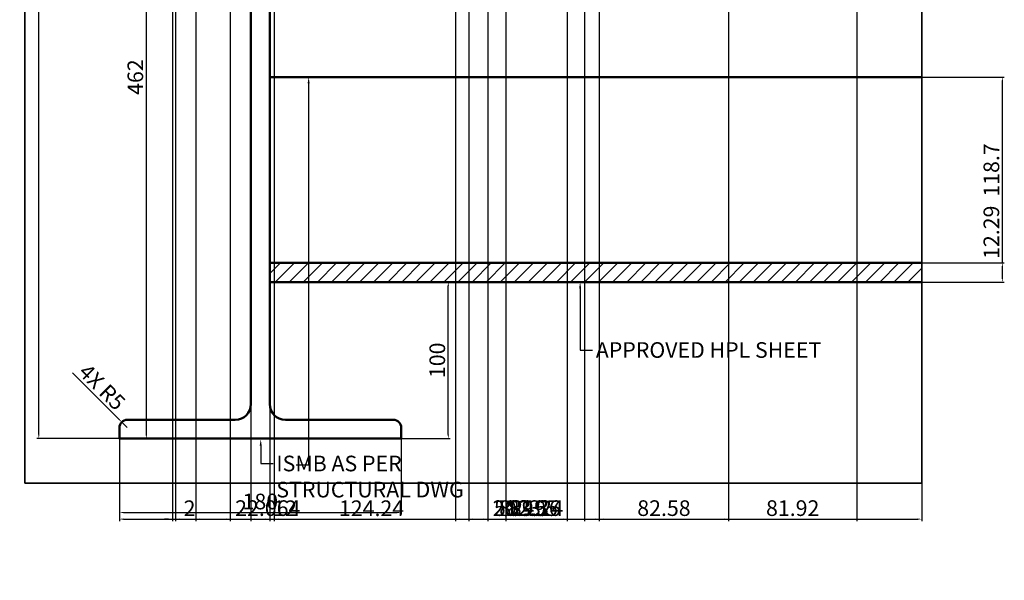
# Model space of a CAD drawing. Units: millimetres. Extents: x 1791 to 2420, y 1225 to 2361.
# Tile 1 of 4: x 1791 to 2420, y 1225 to 1583. Entities that reach past the tile are written whole.
import ezdxf
from ezdxf import colors
from ezdxf.entities.mleader import LeaderData, LeaderLine
from ezdxf.math import Vec2, Vec3

# ---------------------------------------------------------------- set-up
doc = ezdxf.new("R2010")
doc.units = ezdxf.units.MM
for name, color, linetype, lineweight in [('A-ANNO-DIMS', 2, 'Continuous', 18), ('A-ANNO-TEXT', 7, 'Continuous', 18), ('A-ANNO-TTLB', 7, 'Continuous', 35), ('A-DETL-PATT', 8, 'Continuous', 13), ('S-BEAM', 1, 'Continuous', 50)]:
    doc.layers.add(name, color=color, linetype=linetype, lineweight=lineweight)
doc.styles.get("Standard").update_dxf_attribs({"font": 'arial.ttf'})
doc.dimstyles.new('ISO-25', dxfattribs={"dimtxt": 10, "dimasz": 2.5, "dimexe": 1.25, "dimexo": 0.625, "dimtad": 1, "dimdec": 1, "dimtxsty": 'Standard', "dimcen": 2.5, "dimadec": 0, "dimazin": 0, "dimtfac": 1, "dimtdec": 1, "dimtmove": 0, "dimatfit": 3, "dimfxl": 1, "dimarcsym": 0})

# ---------------------------------------------------------------- blocks, each defined once
blk = doc.blocks.new('*D3')
at = {"layer": 'A-ANNO-DIMS', "color": 0, "lineweight": -2, "transparency": 16777216}
for p, q in [((1860.7, 1777.42), (1873.17, 1777.42)), ((1871.92, 1317.92), (1871.92, 1774.92)), ((1860.7, 1315.42), (1873.17, 1315.42))]:
    blk.add_line(p, q, dxfattribs=at)
at = {"layer": 'A-ANNO-DIMS', "color": 0, "transparency": 16777216}
for points in [[(1871.5, 1774.92), (1872.34, 1774.92), (1871.92, 1777.42)], [(1871.5, 1317.92), (1872.34, 1317.92), (1871.92, 1315.42)]]:
    blk.add_solid(points, dxfattribs=at)
at = {"layer": 'Defpoints', "color": 0, "transparency": 16777216}
for p in [(1860.08, 1777.42), (1871.92, 1777.42), (1860.08, 1315.42)]:
    blk.add_point(p, dxfattribs=at)
at = {"layer": 'A-ANNO-DIMS', "color": 0, "transparency": 16777216, "insert": (1866.19, 1546.42), "char_height": 10, "attachment_point": 5, "rotation": 90}
blk.add_mtext('462', dxfattribs=at)
blk = doc.blocks.new('*D5')
at = {"layer": 'A-ANNO-DIMS', "color": 0, "lineweight": -2, "transparency": 16777216}
for p, q in [((1854.73, 1314.8), (1854.73, 1266.91)), ((2034.73, 1314.8), (2034.73, 1266.91)), ((1857.23, 1268.16), (2032.23, 1268.16))]:
    blk.add_line(p, q, dxfattribs=at)
at = {"layer": 'A-ANNO-DIMS', "color": 0, "transparency": 16777216}
for points in [[(1857.23, 1268.58), (1857.23, 1267.74), (1854.73, 1268.16)], [(2032.23, 1268.58), (2032.23, 1267.74), (2034.73, 1268.16)]]:
    blk.add_solid(points, dxfattribs=at)
at = {"layer": 'Defpoints', "color": 0, "transparency": 16777216}
for p in [(1854.73, 1315.42), (2034.73, 1315.42), (2034.73, 1268.16)]:
    blk.add_point(p, dxfattribs=at)
at = {"layer": 'A-ANNO-DIMS', "color": 0, "transparency": 16777216, "insert": (1944.73, 1273.89), "char_height": 10, "attachment_point": 5}
blk.add_mtext('180', dxfattribs=at)
blk = doc.blocks.new('*D6')
at = {"layer": 'A-ANNO-DIMS', "color": 0, "lineweight": -2, "transparency": 16777216}
for p, q in [((2035.35, 1415.42), (2066.04, 1415.42)), ((2064.79, 1317.92), (2064.79, 1412.92)), ((2035.35, 1315.42), (2066.04, 1315.42))]:
    blk.add_line(p, q, dxfattribs=at)
at = {"layer": 'A-ANNO-DIMS', "color": 0, "transparency": 16777216}
for points in [[(2064.38, 1412.92), (2065.21, 1412.92), (2064.79, 1415.42)], [(2064.38, 1317.92), (2065.21, 1317.92), (2064.79, 1315.42)]]:
    blk.add_solid(points, dxfattribs=at)
at = {"layer": 'Defpoints', "color": 0, "transparency": 16777216}
for p in [(2034.73, 1415.42), (2064.79, 1415.42), (2034.73, 1315.42)]:
    blk.add_point(p, dxfattribs=at)
at = {"layer": 'A-ANNO-DIMS', "color": 0, "transparency": 16777216, "insert": (2059.06, 1365.42), "char_height": 10, "attachment_point": 5, "rotation": 90}
blk.add_mtext('100', dxfattribs=at)
blk = doc.blocks.new('*D10')
at = {"layer": 'A-ANNO-DIMS', "color": 0, "lineweight": -2, "transparency": 16777216}
for p, q in [((2367.22, 1414.8), (2367.22, 1262.67)), ((1854.73, 1314.8), (1854.73, 1262.67)), ((1857.23, 1263.92), (2364.72, 1263.92))]:
    blk.add_line(p, q, dxfattribs=at)
at = {"layer": 'A-ANNO-DIMS', "color": 0, "transparency": 16777216}
for points in [[(1857.23, 1264.34), (1857.23, 1263.5), (1854.73, 1263.92)], [(2364.72, 1264.34), (2364.72, 1263.5), (2367.22, 1263.92)]]:
    blk.add_solid(points, dxfattribs=at)
at = {"layer": 'Defpoints', "color": 0, "transparency": 16777216}
for p in [(2367.22, 1415.42), (1854.73, 1315.42), (2367.22, 1263.92)]:
    blk.add_point(p, dxfattribs=at)
at = {"layer": 'A-ANNO-DIMS', "color": 0, "transparency": 16777216, "insert": (2110.97, 1269.65), "char_height": 10, "attachment_point": 5}
blk.add_mtext('512.5', dxfattribs=at)
blk = doc.blocks.new('*D11')
at = {"layer": 'A-ANNO-DIMS', "color": 0, "lineweight": -2, "transparency": 16777216}
for p, q in [((1894.37, 2284.98), (1801.98, 2284.98)), ((1803.23, 1317.92), (1803.23, 2282.48)), ((1854.1, 1315.42), (1801.98, 1315.42))]:
    blk.add_line(p, q, dxfattribs=at)
at = {"layer": 'A-ANNO-DIMS', "color": 0, "transparency": 16777216}
for points in [[(1802.81, 2282.48), (1803.64, 2282.48), (1803.23, 2284.98)], [(1802.81, 1317.92), (1803.64, 1317.92), (1803.23, 1315.42)]]:
    blk.add_solid(points, dxfattribs=at)
at = {"layer": 'Defpoints', "color": 0, "transparency": 16777216}
for p in [(1803.23, 2284.98), (1895, 2284.98), (1854.73, 1315.42)]:
    blk.add_point(p, dxfattribs=at)
at = {"layer": 'A-ANNO-DIMS', "color": 0, "transparency": 16777216, "insert": (1797.5, 1800.2), "char_height": 10, "attachment_point": 5, "rotation": 90}
blk.add_mtext('969.6', dxfattribs=at)
blk = doc.blocks.new('*D16')
at = {"layer": 'A-ANNO-DIMS', "color": 0, "lineweight": -2, "transparency": 16777216}
for p, q in [((1888.61, 1776.8), (1888.61, 1262.67)), ((1890.61, 1778.8), (1890.61, 1262.67)), ((1886.11, 1263.92), (1883.61, 1263.92)), ((1888.61, 1263.92), (1890.61, 1263.92)), ((1893.11, 1263.92), (1903.49, 1263.92))]:
    blk.add_line(p, q, dxfattribs=at)
at = {"layer": 'A-ANNO-DIMS', "color": 0, "transparency": 16777216}
for points in [[(1886.11, 1264.34), (1886.11, 1263.5), (1888.61, 1263.92)], [(1893.11, 1264.34), (1893.11, 1263.5), (1890.61, 1263.92)]]:
    blk.add_solid(points, dxfattribs=at)
at = {"layer": 'Defpoints', "color": 0, "transparency": 16777216}
for p in [(1888.61, 1777.42), (1890.61, 1779.42), (1890.61, 1263.92)]:
    blk.add_point(p, dxfattribs=at)
at = {"layer": 'A-ANNO-DIMS', "color": 0, "transparency": 16777216, "insert": (1899.55, 1269.57), "char_height": 10, "attachment_point": 5}
blk.add_mtext('2', dxfattribs=at)
blk = doc.blocks.new('*D17')
at = {"layer": 'A-ANNO-DIMS', "color": 0, "lineweight": -2, "transparency": 16777216}
for p, q in [((1903.46, 1791.65), (1903.46, 1262.67)), ((1925.53, 1791.65), (1925.53, 1262.67)), ((1905.96, 1263.92), (1923.03, 1263.92)), ((1925.53, 1263.92), (1970.92, 1263.92))]:
    blk.add_line(p, q, dxfattribs=at)
at = {"layer": 'A-ANNO-DIMS', "color": 0, "transparency": 16777216}
for points in [[(1905.96, 1264.34), (1905.96, 1263.5), (1903.46, 1263.92)], [(1923.03, 1264.34), (1923.03, 1263.5), (1925.53, 1263.92)]]:
    blk.add_solid(points, dxfattribs=at)
at = {"layer": 'Defpoints', "color": 0, "transparency": 16777216}
for p in [(1903.46, 1792.27), (1925.53, 1792.27), (1925.53, 1263.92)]:
    blk.add_point(p, dxfattribs=at)
at = {"layer": 'A-ANNO-DIMS', "color": 0, "transparency": 16777216, "insert": (1949.47, 1269.65), "char_height": 10, "attachment_point": 5}
blk.add_mtext('22.064', dxfattribs=at)
blk = doc.blocks.new('*D20')
at = {"layer": 'A-ANNO-DIMS', "color": 0, "lineweight": -2, "transparency": 16777216}
for p, q in [((1938.73, 1336.8), (1938.73, 1262.67)), ((1950.73, 1336.8), (1950.73, 1262.67)), ((1941.23, 1263.92), (1948.23, 1263.92)), ((1950.73, 1263.92), (1967.76, 1263.92))]:
    blk.add_line(p, q, dxfattribs=at)
at = {"layer": 'A-ANNO-DIMS', "color": 0, "transparency": 16777216}
for points in [[(1941.23, 1264.34), (1941.23, 1263.5), (1938.73, 1263.92)], [(1948.23, 1264.34), (1948.23, 1263.5), (1950.73, 1263.92)]]:
    blk.add_solid(points, dxfattribs=at)
at = {"layer": 'Defpoints', "color": 0, "transparency": 16777216}
for p in [(1938.73, 1337.42), (1950.73, 1337.42), (1950.73, 1263.92)]:
    blk.add_point(p, dxfattribs=at)
at = {"layer": 'A-ANNO-DIMS', "color": 0, "transparency": 16777216, "insert": (1960.49, 1269.57), "char_height": 10, "attachment_point": 5}
blk.add_mtext('12', dxfattribs=at)
blk = doc.blocks.new('*D29')
at = {"layer": 'A-ANNO-DIMS', "color": 0, "lineweight": -2, "transparency": 16777216}
for p, q in [((2069.49, 1724.43), (2069.49, 1262.67)), ((2089.99, 1724.43), (2089.99, 1262.67)), ((2071.99, 1263.92), (2087.49, 1263.92)), ((2089.99, 1263.92), (2135.5, 1263.92))]:
    blk.add_line(p, q, dxfattribs=at)
at = {"layer": 'A-ANNO-DIMS', "color": 0, "transparency": 16777216}
for points in [[(2071.99, 1264.34), (2071.99, 1263.5), (2069.49, 1263.92)], [(2087.49, 1264.34), (2087.49, 1263.5), (2089.99, 1263.92)]]:
    blk.add_solid(points, dxfattribs=at)
at = {"layer": 'Defpoints', "color": 0, "transparency": 16777216}
for p in [(2069.49, 1725.06), (2089.99, 1725.06), (2089.99, 1263.92)]:
    blk.add_point(p, dxfattribs=at)
at = {"layer": 'A-ANNO-DIMS', "color": 0, "transparency": 16777216, "insert": (2113.99, 1269.65), "char_height": 10, "attachment_point": 5}
blk.add_mtext('20.495', dxfattribs=at)
blk = doc.blocks.new('*D30')
at = {"layer": 'A-ANNO-DIMS', "color": 0, "lineweight": -2, "transparency": 16777216}
for p, q in [((2069.49, 1724.43), (2069.49, 1262.67)), ((2151.78, 1724.43), (2151.78, 1262.67)), ((2071.99, 1263.92), (2149.28, 1263.92))]:
    blk.add_line(p, q, dxfattribs=at)
at = {"layer": 'A-ANNO-DIMS', "color": 0, "transparency": 16777216}
for points in [[(2071.99, 1264.34), (2071.99, 1263.5), (2069.49, 1263.92)], [(2149.28, 1264.34), (2149.28, 1263.5), (2151.78, 1263.92)]]:
    blk.add_solid(points, dxfattribs=at)
at = {"layer": 'Defpoints', "color": 0, "transparency": 16777216}
for p in [(2069.49, 1725.06), (2151.78, 1725.06), (2151.78, 1263.92)]:
    blk.add_point(p, dxfattribs=at)
at = {"layer": 'A-ANNO-DIMS', "color": 0, "transparency": 16777216, "insert": (2110.64, 1269.65), "char_height": 10, "attachment_point": 5}
blk.add_mtext('82.3', dxfattribs=at)
blk = doc.blocks.new('*D31')
at = {"layer": 'A-ANNO-DIMS', "color": 0, "lineweight": -2, "transparency": 16777216}
for p, q in [((2101.6, 1745.71), (2101.6, 1262.67)), ((2140.84, 1745.71), (2140.84, 1262.67)), ((2104.1, 1263.92), (2138.34, 1263.92))]:
    blk.add_line(p, q, dxfattribs=at)
at = {"layer": 'A-ANNO-DIMS', "color": 0, "transparency": 16777216}
for points in [[(2104.1, 1264.34), (2104.1, 1263.5), (2101.6, 1263.92)], [(2138.34, 1264.34), (2138.34, 1263.5), (2140.84, 1263.92)]]:
    blk.add_solid(points, dxfattribs=at)
at = {"layer": 'Defpoints', "color": 0, "transparency": 16777216}
for p in [(2101.6, 1746.33), (2140.84, 1746.33), (2140.84, 1263.92)]:
    blk.add_point(p, dxfattribs=at)
at = {"layer": 'A-ANNO-DIMS', "color": 0, "transparency": 16777216, "insert": (2121.22, 1269.65), "char_height": 10, "attachment_point": 5}
blk.add_mtext('39.24', dxfattribs=at)
blk = doc.blocks.new('*D32')
at = {"layer": 'A-ANNO-DIMS', "color": 0, "lineweight": -2, "transparency": 16777216}
for p, q in [((1953.66, 1761.87), (1953.66, 1262.67)), ((2077.9, 1766.79), (2077.9, 1262.67)), ((1956.16, 1263.92), (2075.4, 1263.92))]:
    blk.add_line(p, q, dxfattribs=at)
at = {"layer": 'A-ANNO-DIMS', "color": 0, "transparency": 16777216}
for points in [[(1956.16, 1264.34), (1956.16, 1263.5), (1953.66, 1263.92)], [(2075.4, 1264.34), (2075.4, 1263.5), (2077.9, 1263.92)]]:
    blk.add_solid(points, dxfattribs=at)
at = {"layer": 'Defpoints', "color": 0, "transparency": 16777216}
for p in [(2077.9, 1767.42), (1953.66, 1762.49), (2077.9, 1263.92)]:
    blk.add_point(p, dxfattribs=at)
at = {"layer": 'A-ANNO-DIMS', "color": 0, "transparency": 16777216, "insert": (2015.78, 1269.57), "char_height": 10, "attachment_point": 5}
blk.add_mtext('124.24', dxfattribs=at)
blk = doc.blocks.new('*D33')
at = {"layer": 'A-ANNO-DIMS', "color": 0, "lineweight": -2, "transparency": 16777216}
for p, q in [((2077.9, 1766.79), (2077.9, 1262.67)), ((2161.26, 1766.79), (2161.26, 1262.67)), ((2080.4, 1263.92), (2158.76, 1263.92))]:
    blk.add_line(p, q, dxfattribs=at)
at = {"layer": 'A-ANNO-DIMS', "color": 0, "transparency": 16777216}
for points in [[(2080.4, 1264.34), (2080.4, 1263.5), (2077.9, 1263.92)], [(2158.76, 1264.34), (2158.76, 1263.5), (2161.26, 1263.92)]]:
    blk.add_solid(points, dxfattribs=at)
at = {"layer": 'Defpoints', "color": 0, "transparency": 16777216}
for p in [(2077.9, 1767.42), (2161.26, 1767.42), (2161.26, 1263.92)]:
    blk.add_point(p, dxfattribs=at)
at = {"layer": 'A-ANNO-DIMS', "color": 0, "transparency": 16777216, "insert": (2119.58, 1269.65), "char_height": 10, "attachment_point": 5}
blk.add_mtext('83.36', dxfattribs=at)
blk = doc.blocks.new('*D34')
at = {"layer": 'A-ANNO-DIMS', "color": 0, "lineweight": -2, "transparency": 16777216}
for p, q in [((2161.26, 1766.79), (2161.26, 1262.67)), ((2243.84, 1766.79), (2243.84, 1262.67)), ((2163.76, 1263.92), (2241.34, 1263.92))]:
    blk.add_line(p, q, dxfattribs=at)
at = {"layer": 'A-ANNO-DIMS', "color": 0, "transparency": 16777216}
for points in [[(2163.76, 1264.34), (2163.76, 1263.5), (2161.26, 1263.92)], [(2241.34, 1264.34), (2241.34, 1263.5), (2243.84, 1263.92)]]:
    blk.add_solid(points, dxfattribs=at)
at = {"layer": 'Defpoints', "color": 0, "transparency": 16777216}
for p in [(2161.26, 1767.42), (2243.84, 1767.42), (2243.84, 1263.92)]:
    blk.add_point(p, dxfattribs=at)
at = {"layer": 'A-ANNO-DIMS', "color": 0, "transparency": 16777216, "insert": (2202.55, 1269.65), "char_height": 10, "attachment_point": 5}
blk.add_mtext('82.58', dxfattribs=at)
blk = doc.blocks.new('*D35')
at = {"layer": 'A-ANNO-DIMS', "color": 0, "lineweight": -2, "transparency": 16777216}
for p, q in [((2243.84, 1766.79), (2243.84, 1262.67)), ((2325.75, 1766.79), (2325.75, 1262.67)), ((2246.34, 1263.92), (2323.25, 1263.92))]:
    blk.add_line(p, q, dxfattribs=at)
at = {"layer": 'A-ANNO-DIMS', "color": 0, "transparency": 16777216}
for points in [[(2246.34, 1264.34), (2246.34, 1263.5), (2243.84, 1263.92)], [(2323.25, 1264.34), (2323.25, 1263.5), (2325.75, 1263.92)]]:
    blk.add_solid(points, dxfattribs=at)
at = {"layer": 'Defpoints', "color": 0, "transparency": 16777216}
for p in [(2243.84, 1767.42), (2325.75, 1767.42), (2325.75, 1263.92)]:
    blk.add_point(p, dxfattribs=at)
at = {"layer": 'A-ANNO-DIMS', "color": 0, "transparency": 16777216, "insert": (2284.8, 1269.65), "char_height": 10, "attachment_point": 5}
blk.add_mtext('81.92', dxfattribs=at)
blk = doc.blocks.new('*D36')
at = {"layer": 'A-ANNO-DIMS', "color": 0, "lineweight": -2, "transparency": 16777216}
for p, q in [((2367.84, 1546.42), (2419.97, 1546.42)), ((2418.72, 1430.21), (2418.72, 1543.92)), ((2367.84, 1427.71), (2419.97, 1427.71))]:
    blk.add_line(p, q, dxfattribs=at)
at = {"layer": 'A-ANNO-DIMS', "color": 0, "transparency": 16777216}
for points in [[(2418.3, 1543.92), (2419.13, 1543.92), (2418.72, 1546.42)], [(2418.3, 1430.21), (2419.13, 1430.21), (2418.72, 1427.71)]]:
    blk.add_solid(points, dxfattribs=at)
at = {"layer": 'Defpoints', "color": 0, "transparency": 16777216}
for p in [(2367.22, 1546.42), (2418.72, 1546.42), (2367.22, 1427.71)]:
    blk.add_point(p, dxfattribs=at)
at = {"layer": 'A-ANNO-DIMS', "color": 0, "transparency": 16777216, "insert": (2412.99, 1487.06), "char_height": 10, "attachment_point": 5, "rotation": 90}
blk.add_mtext('118.7', dxfattribs=at)
blk = doc.blocks.new('*D37')
at = {"layer": 'A-ANNO-DIMS', "color": 0, "lineweight": -2, "transparency": 16777216}
for p, q in [((2418.72, 1427.71), (2418.72, 1464.28)), ((2367.84, 1427.71), (2419.97, 1427.71)), ((2418.72, 1417.92), (2418.72, 1425.21)), ((2367.84, 1415.42), (2419.97, 1415.42))]:
    blk.add_line(p, q, dxfattribs=at)
at = {"layer": 'A-ANNO-DIMS', "color": 0, "transparency": 16777216}
for points in [[(2418.3, 1425.21), (2419.13, 1425.21), (2418.72, 1427.71)], [(2418.3, 1417.92), (2419.13, 1417.92), (2418.72, 1415.42)]]:
    blk.add_solid(points, dxfattribs=at)
at = {"layer": 'Defpoints', "color": 0, "transparency": 16777216}
for p in [(2367.22, 1427.71), (2418.72, 1427.71), (2367.22, 1415.42)]:
    blk.add_point(p, dxfattribs=at)
at = {"layer": 'A-ANNO-DIMS', "color": 0, "transparency": 16777216, "insert": (2412.99, 1447.25), "char_height": 10, "attachment_point": 5, "rotation": 90}
blk.add_mtext('12.29', dxfattribs=at)
blk = doc.blocks.new('*D39')
at = {"layer": 'A-ANNO-DIMS', "color": 0, "lineweight": -2, "transparency": 16777216}
for p, q in [((1824.84, 1357.31), (1854.42, 1327.72)), ((1859.73, 1322.42), (1856.19, 1325.96))]:
    blk.add_line(p, q, dxfattribs=at)
at = {"layer": 'A-ANNO-DIMS', "color": 0, "transparency": 16777216}
blk.add_solid([(1854.72, 1328.02), (1854.13, 1327.43), (1856.19, 1325.96)], dxfattribs=at)
at = {"layer": 'Defpoints', "color": 0, "transparency": 16777216}
for p in [(1856.19, 1325.96), (1859.73, 1322.42)]:
    blk.add_point(p, dxfattribs=at)
at = {"layer": 'A-ANNO-DIMS', "color": 0, "transparency": 16777216, "insert": (1842.78, 1347.44), "char_height": 10, "attachment_point": 5, "rotation": 315.00466}
blk.add_mtext('4X R5', dxfattribs=at)

msp = doc.modelspace()

# ---------------------------------------------------------------- hatches: boundary and pattern name
at = {"layer": 'A-DETL-PATT'}
h = msp.add_hatch(dxfattribs=at)
h.set_pattern_fill('ANSI31', color=256, scale=2)
h.paths.add_polyline_path([(2367.2176, 1415.4206), (2367.2176, 1427.7094), (1950.727, 1427.7094), (1950.727, 1415.4206)])

# ---------------------------------------------------------------- linework, layer by layer
at = {"layer": 'A-ANNO-TTLB'}
for p, q in [((1794.3467, 1287.0028), (1794.3467, 2307.8191)), ((2367.2176, 2307.8191), (2367.2176, 1287.0028)), ((2367.2176, 1287.0028), (1794.3467, 1287.0028))]:
    msp.add_line(p, q, dxfattribs=at)
at = {"layer": 'S-BEAM'}
for p, q in [((1950.727, 1546.4206), (2367.2176, 1546.4206)), ((1950.727, 1427.7094), (2367.2176, 1427.7094)), ((1950.727, 1415.4206), (2367.2176, 1415.4206))]:
    msp.add_line(p, q, dxfattribs=at)
msp.add_lwpolyline([(1938.727, 1755.4206, 0.41421356), (1928.727, 1765.4206), (1859.727, 1765.4206, -0.41421356), (1854.727, 1770.4206), (1854.727, 1777.4206), (2034.727, 1777.4206), (2034.727, 1770.4206, -0.41421356), (2029.727, 1765.4206), (1960.727, 1765.4206, 0.41421356), (1950.727, 1755.4206), (1950.727, 1337.4206, 0.41421356), (1960.727, 1327.4206), (2029.727, 1327.4206, -0.41421356), (2034.727, 1322.4206), (2034.727, 1315.4206), (1854.727, 1315.4206), (1854.727, 1322.4206, -0.41421356), (1859.727, 1327.4206), (1928.727, 1327.4206, 0.41421356), (1938.727, 1337.4206), (1938.727, 1755.4206)], format="xyb", dxfattribs=at)

# ---------------------------------------------------------------- dimensions: what is measured, and where the dimension line sits
at = {"layer": 'A-ANNO-DIMS'}
for base, p1, p2, override, picture, middle in [((1803.227, 2284.9823), (1854.727, 1315.4206), (1894.9953, 2284.9823), {"dimdec": 1, "dimlfac": 1, "dimrnd": 0, "dimzin": 0, "dimdsep": 46, "dimlunit": 2}, '*D11', (1797.4963, 1800.2015)), ((2418.7176, 1546.4206), (2367.2176, 1427.7094), (2367.2176, 1546.4206), {"dimdec": 1, "dimlfac": 1, "dimrnd": 0, "dimzin": 0, "dimdsep": 46, "dimlunit": 2}, '*D36', (2412.9869, 1487.065)), ((2418.7176, 1427.7094), (2367.2176, 1415.4206), (2367.2176, 1427.7094), {"dimdec": 2, "dimlfac": 1, "dimrnd": 0, "dimzin": 0, "dimdsep": 46, "dimlunit": 2}, '*D37', (2412.9869, 1447.2464))]:
    dim = msp.add_linear_dim(base=base, p1=p1, p2=p2, angle=90, dimstyle='ISO-25', override=override, dxfattribs=at)
    dim.commit()
    dim.dimension.update_dxf_attribs({"geometry": picture, "text_midpoint": middle})
for base, p1, p2, override, picture, middle in [((1925.5277, 1263.9206), (1903.4637, 1792.271), (1925.5277, 1792.271), {"dimdec": 3, "dimlfac": 1, "dimrnd": 0, "dimzin": 0, "dimdsep": 46, "dimlunit": 2}, '*D17', (1949.4746, 1269.6513)), ((1890.6133, 1263.9206), (1888.6133, 1777.4206), (1890.6133, 1779.4206), {"dimdec": 0, "dimlfac": 1, "dimrnd": 0, "dimzin": 0, "dimdsep": 46, "dimlunit": 2}, '*D16', (1899.5501, 1269.566)), ((2077.8995, 1263.9206), (1953.6559, 1762.4917), (2077.8995, 1767.4162), {"dimdec": 2, "dimlfac": 1, "dimrnd": 0, "dimzin": 0, "dimdsep": 46, "dimlunit": 2}, '*D32', (2015.7777, 1269.566)), ((2161.2551, 1263.9206), (2077.8995, 1767.4162), (2161.2551, 1767.4162), {"dimdec": 2, "dimlfac": 1, "dimrnd": 0, "dimzin": 0, "dimdsep": 46, "dimlunit": 2}, '*D33', (2119.5773, 1269.6547)), ((2243.8358, 1263.9206), (2161.2551, 1767.4162), (2243.8358, 1767.4162), {"dimdec": 2, "dimlfac": 1, "dimrnd": 0, "dimzin": 0, "dimdsep": 46, "dimlunit": 2}, '*D34', (2202.5454, 1269.6513)), ((2325.7548, 1263.9206), (2243.8358, 1767.4162), (2325.7548, 1767.4162), {"dimdec": 2, "dimlfac": 1, "dimrnd": 0, "dimzin": 0, "dimdsep": 46, "dimlunit": 2}, '*D35', (2284.7953, 1269.6513)), ((2140.839, 1263.9206), (2101.6014, 1746.3347), (2140.839, 1746.3347), {"dimdec": 2, "dimlfac": 1, "dimrnd": 0, "dimzin": 0, "dimdsep": 46, "dimlunit": 2}, '*D31', (2121.2202, 1269.6547)), ((2089.9858, 1263.9206), (2069.4909, 1725.0563), (2089.9858, 1725.0563), {"dimdec": 3, "dimlfac": 1, "dimrnd": 0, "dimzin": 0, "dimdsep": 46, "dimlunit": 2}, '*D29', (2113.9908, 1269.6513)), ((2151.7847, 1263.9206), (2069.4909, 1725.0563), (2151.7847, 1725.0563), {"dimdec": 1, "dimlfac": 1, "dimrnd": 0, "dimzin": 0, "dimdsep": 46, "dimlunit": 2}, '*D30', (2110.6378, 1269.6547)), ((2367.2176, 1263.9206), (1854.727, 1315.4206), (2367.2176, 1415.4206), {"dimdec": 1, "dimlfac": 1, "dimrnd": 0, "dimzin": 0, "dimdsep": 46, "dimlunit": 2}, '*D10', (2110.9723, 1269.6513)), ((1950.727, 1263.9206), (1938.727, 1337.4206), (1950.727, 1337.4206), {"dimdec": 0, "dimlfac": 1, "dimrnd": 0, "dimzin": 0, "dimdsep": 46, "dimlunit": 2}, '*D20', (1960.4925, 1269.566))]:
    dim = msp.add_linear_dim(base=base, p1=p1, p2=p2, dimstyle='ISO-25', override=override, dxfattribs=at)
    dim.commit()
    dim.dimension.update_dxf_attribs({"geometry": picture, "text_midpoint": middle})
for p1, p2, distance, picture, middle in [((1860.0795, 1315.4206), (1860.0795, 1777.4206), -11.8389, '*D3', (1866.1876, 1546.4206)), ((2034.727, 1315.4206), (2034.727, 1415.4206), -30.0664, '*D6', (2059.0626, 1365.4206)), ((1854.727, 1315.4206), (2034.727, 1315.4206), -47.2602, '*D5', (1944.727, 1273.8911))]:
    dim = msp.add_aligned_dim(p1=p1, p2=p2, distance=distance, dimstyle='ISO-25', override={"dimclrd": 0, "dimclre": 0, "dimclrt": 0}, dxfattribs=at)
    dim.commit()
    dim.dimension.update_dxf_attribs({"geometry": picture, "text_midpoint": middle})
dim = msp.add_radius_dim(center=(1859.727, 1322.4206), mpoint=(1856.1912, 1325.9558), text='4X <>', dimstyle='ISO-25', override={"dimdec": 0, "dimlfac": 1, "dimrnd": 0, "dimzin": 0, "dimdsep": 46, "dimlunit": 2}, dxfattribs=at)
dim.commit()
dim.dimension.update_dxf_attribs({"geometry": '*D39', "text_midpoint": (1842.7829, 1347.4368)})

# ---------------------------------------------------------------- leaders
at = {"layer": 'A-ANNO-TEXT'}
ml = msp.add_multileader_mtext('Standard', dxfattribs=at)
ml.set_content('', color=256)
ml.set_leader_properties()
ml.build(insert=Vec2(0, 0))
ctx = ml.context
ctx.base_point, ctx.plane_origin = Vec3(1963.584, 1298.3257), Vec3(1975.584, 1546.4206)
ctx.text_align_type = 2
notes = []
notes.append((ctx, [(0, (1, 1, 0), (1975.584, 1298.3257), (-1, 0), 8, [(0, [(1975.584, 1546.4206)], 0, [])])]))
ctx.mtext.insert, ctx.mtext.alignment, ctx.mtext.flow_direction = Vec3(1965.584, 1300.3257), 3, 5
ml = msp.add_multileader_mtext('Standard', dxfattribs=at)
ml.set_content('APPROVED HPL SHEET', color=256)
ml.set_leader_properties()
ml.build(insert=Vec2(0, 0))
ctx = ml.context
ctx.base_point, ctx.char_height, ctx.plane_origin = Vec3(2157.0207, 1371.9244), 10, Vec3(2149.0207, 1415.4206)
notes.append((ctx, [(0, (1, 1, 0), (2149.0207, 1371.9244), (1, 0), 8, [(0, [(2149.0207, 1415.4206)], 0, [])])]))
ctx.mtext.insert, ctx.mtext.flow_direction = Vec3(2159.0207, 1377.0097), 5
ml = msp.add_multileader_mtext('Standard', dxfattribs=at)
ml.set_content('ISMB AS PER \\PSTRUCTURAL DWG', color=256)
ml.set_leader_properties()
ml.build(insert=Vec2(0, 0))
ctx = ml.context
ctx.base_point, ctx.char_height, ctx.plane_origin = Vec3(1952.9744, 1299.3745), 10, Vec3(1944.9744, 1314.9149)
notes.append((ctx, [(0, (1, 1, 0), (1944.9744, 1299.3745), (1, 0), 8, [(0, [(1944.9744, 1314.9149)], 0, [])])]))
ctx.mtext.insert, ctx.mtext.flow_direction = Vec3(1954.9744, 1304.4598), 5
for ctx, leaders in notes:
    for number, flags, end, landing, length, lines in leaders:
        leader = LeaderData()
        leader.index, (leader.has_last_leader_line, leader.has_dogleg_vector, leader.attachment_direction) = number, flags
        leader.last_leader_point, leader.dogleg_vector, leader.dogleg_length = Vec3(end), Vec3(landing), length
        for number, points, colour, breaks in lines:
            line = LeaderLine()
            line.index, line.vertices, line.color, line.breaks = number, Vec3.list(points), colors.encode_raw_color(colour), breaks
            leader.lines.append(line)
        ctx.leaders.append(leader)

doc.saveas('drawing.dxf')
